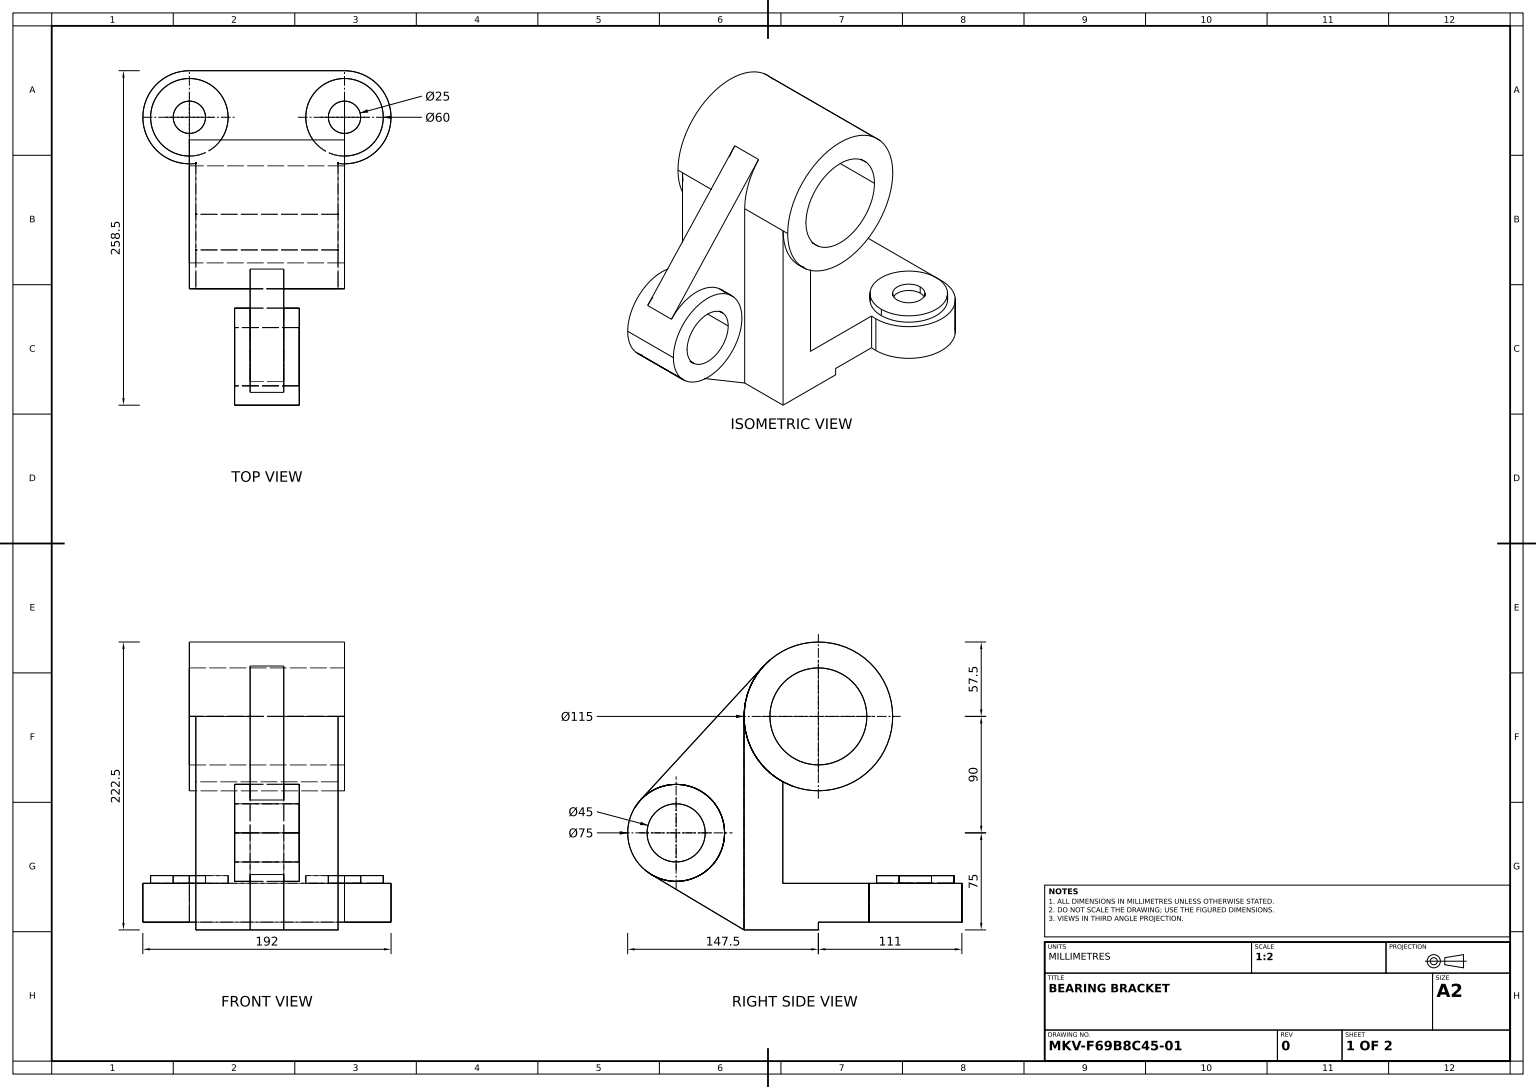
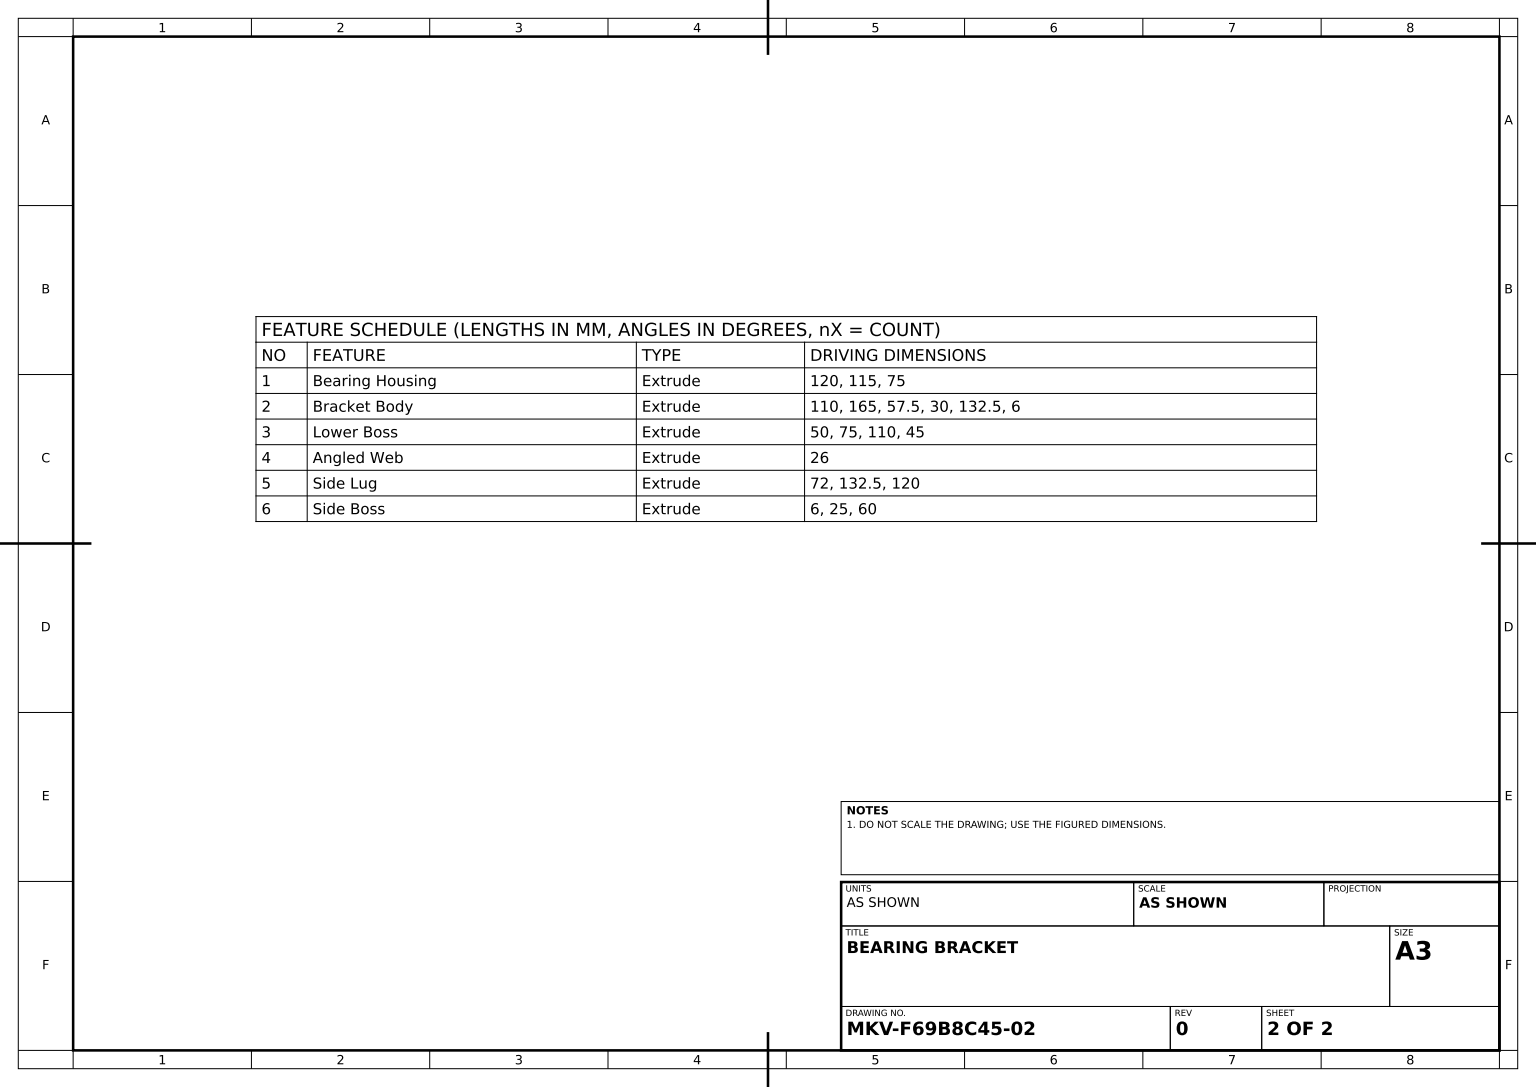
SolidWorks part; units mm, degrees
material "Plain Carbon Steel"
ref_plane "Front Plane" through (0, 0, 0) normal (0, 0, 1) x (1, 0, 0)
ref_plane "Top Plane" through (0, 0, 0) normal (0, 1, 0) x (1, 0, 0)
ref_plane "Right Plane" through (0, 0, 0) normal (1, 0, 0) x (0, 0, -1)
sketch "Bearing Housing Sketch" plane through (0, 0, 0) normal (1, 0, 0) x (0, 0, -1)
  circle A0 centre (0, 0) radius 37.5
  circle A1 centre (0, 0) radius 57.5
  dimension "D1" = 115
  dimension "D2" = 75
extrude "Bearing Housing" add sketch "Bearing Housing Sketch" along normal mid plane 120
sketch "Bracket Body Sketch" plane through (0, 0, 0) normal (1, 0, 0) x (0, 0, -1)
  line L0 (-57.5, 0) -> (-57.5, -165)
  line L1 (-57.5, -165) -> (0, -165)
  line L2 (0, -165) -> (0, -159)
  line L3 (0, -159) -> (75, -159)
  line L4 (75, -159) -> (75, -129)
  line L5 (75, -129) -> (-27.5, -129)
  line L6 (-27.5, -129) -> (-27.5, -50.4975)
  circle A0 centre (0, 0) radius 57.5 construction
  arc A1 (-57.5, 0) -> (-27.5, -50.4975) centre (0, 0) ccw
  dimension "D1" = 165
  dimension "D2" = 57.5
  dimension "D3" = 30
  dimension "D4" = 30
  dimension "D5" = 132.5
  dimension "D6" = 6
extrude "Bracket Body" add sketch "Bracket Body Sketch" along normal mid plane 110
sketch "Lower Boss Sketch" plane through (0, 0, 0) normal (1, 0, 0) x (0, 0, -1)
  line L0 (-57.5, -165) -> (0, -165) construction
  line L2 (-57.5, 0) -> (-57.5, -165) construction
  line L3 (-57.5, 0) -> (-57.5, -165)
  circle A0 centre (-110, -90) radius 37.5
  circle A1 centre (-110, -90) radius 22.5
  dimension "D3" = 45
  dimension "D4" = 75
  dimension "D1" = 75
  dimension "D2" = 110
extrude "Lower Boss" add sketch "Lower Boss Sketch" along normal mid plane 50 separate body contours A0 A1
sketch "Angled Web Sketch" plane through (0, 0, 0) normal (1, 0, 0) x (0, 0, -1)
  line L0 (-57.5, 0) -> (-57.5, -165) construction
  line L1 (-57.5, 0) -> (-57.5, -165)
  line L2 (-137.5943, -64.607) -> (-42.3112, 38.936)
  line L3 (-57.5, -165) -> (-129.2169, -122.2019)
  circle A0 centre (-110, -90) radius 37.5 construction
  circle A2 centre (0, 0) radius 57.5 construction
  arc A3 (-42.3112, 38.936) -> (-57.5, 0) centre (0, 0) ccw
  arc A4 (-129.2169, -122.2019) -> (-137.5943, -64.607) centre (-110, -90) ccw
extrude "Angled Web" add sketch "Angled Web Sketch" along normal mid plane 26
sketch "Side Lug Sketch" plane through (0, -129, 0) normal (0, 1, 0) x (1, 0, 0)
  line L1 (0, 111) -> (0, 155.8148) construction
  line L2 (-60, 111) -> (60, 111)
  line L3 (-55, 75) -> (-55, -27.5) construction
  line L4 (55, 75) -> (55, -27.5) construction
  line L5 (-55, 39.3489) -> (-55, -27.5)
  line L6 (55, 39.3489) -> (55, -27.5)
  line L7 (-55, -27.5) -> (55, -27.5)
  arc A0 (55, 39.3489) -> (60, 111) centre (60, 75) ccw
  arc A1 (-60, 111) -> (-55, 39.3489) centre (-60, 75) ccw
  dimension "D1" = 72
  dimension "D2" = 72
  dimension "D3" = 132.5
  dimension "D4" = 120
extrude "Side Lug" add sketch "Side Lug Sketch" against normal up to surface (30 mm away) up to face at (0, -159, -37.5)
sketch "Side Boss Sketch" plane through (0, -129, 0) normal (0, 1, 0) x (1, 0, 0)
  circle A0 centre (60, 75) radius 12.5
  circle A1 centre (-60, 75) radius 12.5
  circle A2 centre (60, 75) radius 30
  circle A3 centre (-60, 75) radius 30
  dimension "D1" = 25
  dimension "D2" = 25
  dimension "D3" = 60
  dimension "D4" = 60
extrude "Side Boss" add sketch "Side Boss Sketch" along normal blind 6
